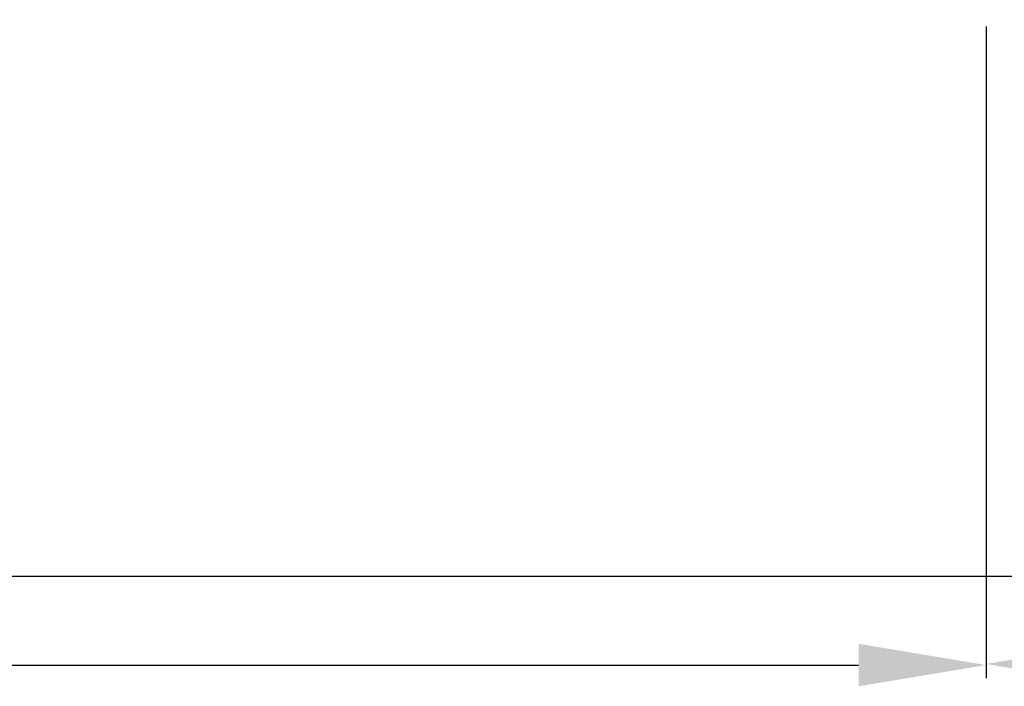
# Model space of a CAD drawing. Units: inches. Extents: x 2083 to 3317, y 1141 to 2115.
# Tile 109 of 256: x 2772 to 2865, y 1201 to 1263. Entities that reach past the tile are written whole.
import ezdxf

# ---------------------------------------------------------------- set-up
doc = ezdxf.new("R2010")
doc.units = ezdxf.units.IN
doc.layers.add('A-ANNO-DIMS', color=2, linetype='Continuous', lineweight=18)
doc.styles.get("Standard").update_dxf_attribs({"font": 'arial.ttf'})
doc.dimstyles.new('ISO-25', dxfattribs={"dimtxt": 12, "dimasz": 12, "dimexe": 1.25, "dimexo": 0.625, "dimtad": 1, "dimlunit": 3, "dimtxsty": 'Standard', "dimcen": 2.5, "dimadec": 0, "dimazin": 0, "dimtfac": 1, "dimtmove": 0, "dimatfit": 3, "dimfxl": 1, "dimarcsym": 0})

# ---------------------------------------------------------------- blocks, each defined once
blk = doc.blocks.new('*D10')
at = {"layer": 'A-ANNO-DIMS', "color": 0, "lineweight": -2, "transparency": 16777216}
for p, q in [((2862.96, 1262.636), (2862.96, 1201.384)), ((3126.96, 1262.636), (3126.96, 1201.384)), ((2874.96, 1202.634), (3114.96, 1202.634))]:
    blk.add_line(p, q, dxfattribs=at)
at = {"layer": 'A-ANNO-DIMS', "color": 0, "transparency": 16777216}
for points in [[(2874.96, 1204.634), (2874.96, 1200.634), (2862.96, 1202.634)], [(3114.96, 1204.634), (3114.96, 1200.634), (3126.96, 1202.634)]]:
    blk.add_solid(points, dxfattribs=at)
at = {"layer": 'Defpoints', "color": 0, "transparency": 16777216}
for p in [(2862.96, 1263.261), (3126.96, 1263.261), (3126.96, 1202.634)]:
    blk.add_point(p, dxfattribs=at)
at = {"layer": 'A-ANNO-DIMS', "color": 0, "transparency": 16777216, "insert": (2994.96, 1209.284), "char_height": 12, "attachment_point": 5}
blk.add_mtext("22'", dxfattribs=at)
blk = doc.blocks.new('*D11')
at = {"layer": 'A-ANNO-DIMS', "color": 0, "lineweight": -2, "transparency": 16777216}
for p, q in [((2544.96, 1262.636), (2544.96, 1201.284)), ((2862.96, 1262.636), (2862.96, 1201.284)), ((2556.96, 1202.534), (2850.96, 1202.534))]:
    blk.add_line(p, q, dxfattribs=at)
at = {"layer": 'A-ANNO-DIMS', "color": 0, "transparency": 16777216}
for points in [[(2556.96, 1204.534), (2556.96, 1200.534), (2544.96, 1202.534)], [(2850.96, 1204.534), (2850.96, 1200.534), (2862.96, 1202.534)]]:
    blk.add_solid(points, dxfattribs=at)
at = {"layer": 'Defpoints', "color": 0, "transparency": 16777216}
for p in [(2544.96, 1263.261), (2862.96, 1263.261), (2862.96, 1202.534)]:
    blk.add_point(p, dxfattribs=at)
at = {"layer": 'A-ANNO-DIMS', "color": 0, "transparency": 16777216, "insert": (2703.96, 1209.286), "char_height": 12, "attachment_point": 5}
blk.add_mtext('26\'-6"', dxfattribs=at)
blk = doc.blocks.new('*D26')
at = {"layer": 'A-ANNO-DIMS', "color": 0, "lineweight": -2, "transparency": 16777216}
for p, q in [((3088.986, 1274.915), (3088.986, 1270.952)), ((3111.24, 1274.915), (3111.24, 1270.952)), ((3076.986, 1272.202), (2840.262, 1272.202)), ((3111.24, 1272.202), (3088.986, 1272.202)), ((3123.24, 1272.202), (3135.24, 1272.202))]:
    blk.add_line(p, q, dxfattribs=at)
at = {"layer": 'A-ANNO-DIMS', "color": 0, "transparency": 16777216}
for points in [[(3076.986, 1274.202), (3076.986, 1270.202), (3088.986, 1272.202)], [(3123.24, 1274.202), (3123.24, 1270.202), (3111.24, 1272.202)]]:
    blk.add_solid(points, dxfattribs=at)
at = {"layer": 'Defpoints', "color": 0, "transparency": 16777216}
for p in [(3088.986, 1275.54), (3111.24, 1275.54), (3088.986, 1272.202)]:
    blk.add_point(p, dxfattribs=at)
at = {"layer": 'A-ANNO-DIMS', "color": 0, "transparency": 16777216, "insert": (2952.624, 1279.032), "char_height": 12, "attachment_point": 5}
blk.add_mtext('NIGHTSTAND 1\'-10 1/2" TYP.', dxfattribs=at)
blk = doc.blocks.new('*D34')
at = {"layer": 'A-ANNO-DIMS', "color": 0, "lineweight": -2, "transparency": 16777216}
for p, q in [((2226.96, 1262.636), (2226.96, 1209.661)), ((3126.96, 1262.636), (3126.96, 1209.661)), ((2238.96, 1210.911), (3114.96, 1210.911))]:
    blk.add_line(p, q, dxfattribs=at)
at = {"layer": 'A-ANNO-DIMS', "color": 0, "transparency": 16777216}
for points in [[(2238.96, 1212.911), (2238.96, 1208.911), (2226.96, 1210.911)], [(3114.96, 1212.911), (3114.96, 1208.911), (3126.96, 1210.911)]]:
    blk.add_solid(points, dxfattribs=at)
at = {"layer": 'Defpoints', "color": 0, "transparency": 16777216}
for p in [(2226.96, 1263.261), (3126.96, 1263.261), (3126.96, 1210.911)]:
    blk.add_point(p, dxfattribs=at)
at = {"layer": 'A-ANNO-DIMS', "color": 0, "transparency": 16777216, "insert": (2676.96, 1217.663), "char_height": 12, "attachment_point": 5}
blk.add_mtext('75\'-0"', dxfattribs=at)

msp = doc.modelspace()

# ---------------------------------------------------------------- dimensions: what is measured, and where the dimension line sits
at = {"layer": 'A-ANNO-DIMS'}
dim = msp.add_linear_dim(base=(3088.986, 1272.202), p1=(3111.24, 1275.54), p2=(3088.986, 1275.54), angle=180, text='NIGHTSTAND <> TYP.', dimstyle='ISO-25', override={"dimdec": 1, "dimlfac": 1, "dimrnd": 0, "dimzin": 1, "dimdsep": 46, "dimlunit": 4, "dimfrac": 2}, dxfattribs=at)
dim.commit()
dim.dimension.update_dxf_attribs({"geometry": '*D26', "text_midpoint": (2952.624, 1279.032)})
for base, p1, p2, override, picture, middle in [((3126.96, 1210.911), (2226.96, 1263.261), (3126.96, 1263.261), {"dimdec": 1, "dimlfac": 1, "dimrnd": 0, "dimzin": 1, "dimdsep": 46, "dimlunit": 4, "dimfrac": 2}, '*D34', (2676.96, 1217.663)), ((2862.96, 1202.534), (2544.96, 1263.261), (2862.96, 1263.261), {"dimclrd": 0, "dimclre": 0, "dimclrt": 0}, '*D11', (2703.96, 1209.286)), ((3126.96, 1202.634), (2862.96, 1263.261), (3126.96, 1263.261), {"dimclrd": 0, "dimclre": 0, "dimclrt": 0}, '*D10', (2994.96, 1209.284))]:
    dim = msp.add_linear_dim(base=base, p1=p1, p2=p2, dimstyle='ISO-25', override=override, dxfattribs=at)
    dim.commit()
    dim.dimension.update_dxf_attribs({"geometry": picture, "text_midpoint": middle})

doc.saveas('drawing.dxf')
